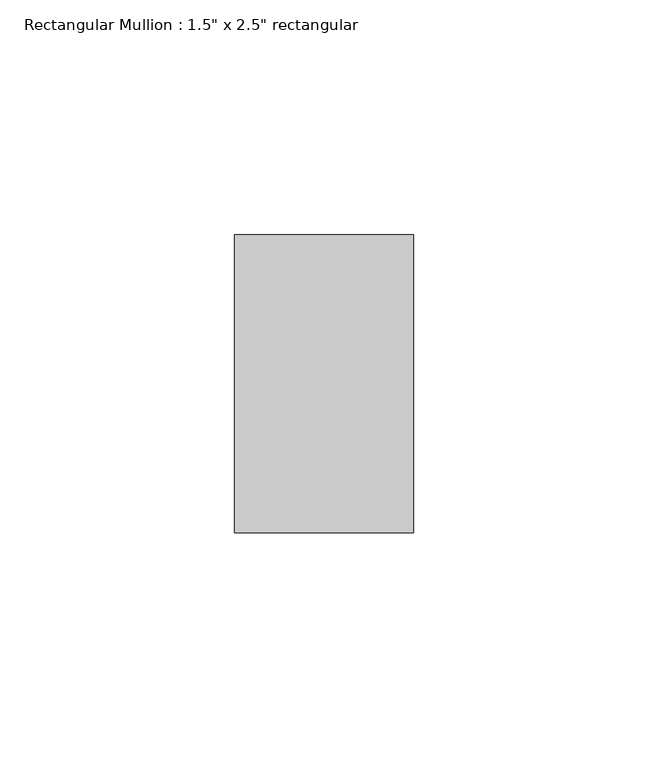
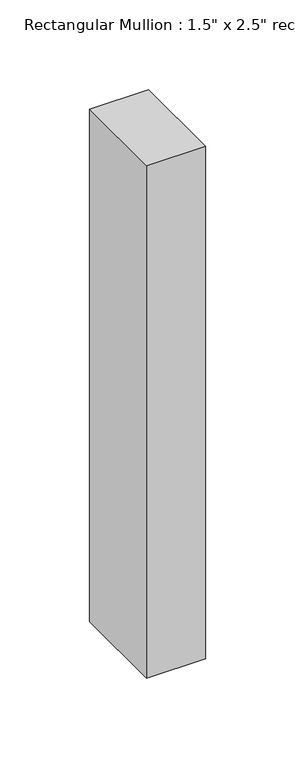
"""IFC4 building model written with IfcOpenShell, lengths in millimetres: member geometry."""

from ifc_helpers import new_model, si_unit, frame, origin, place, context, project, spatial, polyline, outline, extrude, source, transform, mapped, element, save


def member_4cd326a7(model_context):
    return source(origin(), model_context, "Body", "SweptSolid", [
        extrude(outline(polyline([(19.05, 31.75), (19.05, -31.75), (-19.05, -31.75), (-19.05, 31.75), (19.05, 31.75)])), frame((0.0, 0.0, -349.25), z_axis=(0.0, 0.0, 1.0), x_axis=(1.0, 0.0, 0.0)), (0.0, 0.0, 1.0), 349.25),
    ])


if __name__ == "__main__":
    model = new_model("IFC4")
    model_context = context("Model", 3, world=origin())
    ifc_project = project(units=[si_unit("LENGTHUNIT", "METRE", prefix="MILLI")], contexts=[model_context])
    site = spatial("IfcSite", under=ifc_project)
    building = spatial("IfcBuilding", under=site)
    placement = place(None, origin())
    member_shape = member_4cd326a7(model_context)
    element("IfcMember", 1, ObjectType="Rectangular Mullion : 1.5\" x 2.5\" rectangular", at=placement, inside=building, context=model_context, shape_type="MappedRepresentation", body=[
        mapped(member_shape, transform((0.0, 0.0, 0.0), x_axis=(1.0, 0.0, 0.0), y_axis=(0.0, 1.0, 0.0), z_axis=(0.0, 0.0, 1.0))),
    ])
    save(model, "model.ifc")

# Revit data of these elements
# Type "Rectangular Mullion : 1.5\" x 2.5\" rectangular"
#   built-in parameter 1007304 = 0.208333 (stored number, unit not read)
#   built-in parameter 1007301 = 0.0625 (stored number, unit not read)
#   built-in parameter 1007300 = 0.0625 (stored number, unit not read)
# Element 1 (IfcMember, "Rectangular Mullion : 1.5\" x 2.5\" rectangular")
#   Materials on its faces: "Damp-proofing"
# Materials
#   "Damp-proofing": class "Generic", colour RGB 127 127 127, transparency 0, Description = "Damp-proofing", Cost = 0
